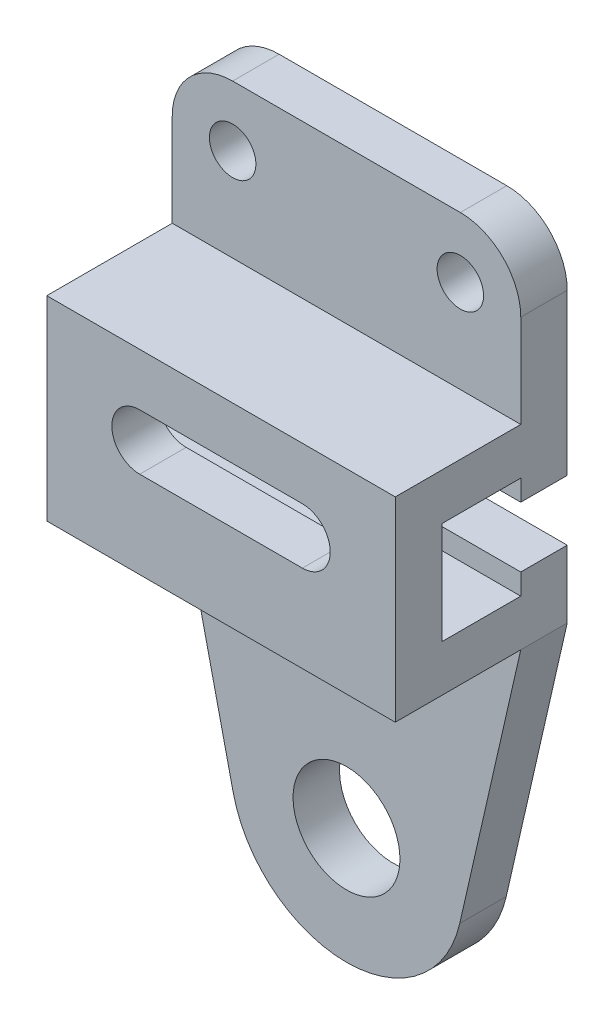
ISO-10303-21;
HEADER;
FILE_DESCRIPTION(('STEP AP214'),'2;1');
FILE_NAME('part.step','',(''),(''),'','','');
FILE_SCHEMA(('AUTOMOTIVE_DESIGN { 1 0 10303 214 1 1 1 1 }'));
ENDSEC;
DATA;
#1=APPLICATION_CONTEXT('core data for automotive mechanical design processes');
#2=APPLICATION_PROTOCOL_DEFINITION('international standard','automotive_design',2000,#1);
#3=PRODUCT_CONTEXT('',#1,'mechanical');
#4=PRODUCT('Part','Part','',(#3));
#5=PRODUCT_RELATED_PRODUCT_CATEGORY('part','',(#4));
#6=PRODUCT_DEFINITION_FORMATION('','',#4);
#7=PRODUCT_DEFINITION_CONTEXT('part definition',#1,'design');
#8=PRODUCT_DEFINITION('design','',#6,#7);
#9=PRODUCT_DEFINITION_SHAPE('','',#8);
#10=(LENGTH_UNIT() NAMED_UNIT(*) SI_UNIT(.MILLI.,.METRE.));
#11=(NAMED_UNIT(*) PLANE_ANGLE_UNIT() SI_UNIT($,.RADIAN.));
#12=(NAMED_UNIT(*) SI_UNIT($,.STERADIAN.) SOLID_ANGLE_UNIT());
#13=UNCERTAINTY_MEASURE_WITH_UNIT(LENGTH_MEASURE(1.E-05),#10,'distance_accuracy_value','');
#14=(GEOMETRIC_REPRESENTATION_CONTEXT(3) GLOBAL_UNCERTAINTY_ASSIGNED_CONTEXT((#13)) GLOBAL_UNIT_ASSIGNED_CONTEXT((#10,
#11,#12)) REPRESENTATION_CONTEXT('',''));
#15=CARTESIAN_POINT('',(0.,0.,0.));
#16=DIRECTION('',(0.,0.,1.));
#17=DIRECTION('',(1.,0.,0.));
#18=AXIS2_PLACEMENT_3D('',#15,#16,#17);
#19=CARTESIAN_POINT('',(0.,63.5,37.));
#20=DIRECTION('',(0.,1.,0.));
#21=DIRECTION('',(0.,0.,1.));
#22=AXIS2_PLACEMENT_3D('',#19,#20,#21);
#23=PLANE('',#22);
#24=DIRECTION('',(0.,0.,-1.));
#25=VECTOR('',#24,1.);
#26=CARTESIAN_POINT('',(-24.4999999999999,63.5,37.));
#27=LINE('',#26,#25);
#28=CARTESIAN_POINT('',(-24.5,63.5,10.));
#29=VERTEX_POINT('',#28);
#30=CARTESIAN_POINT('',(-24.4999999999999,63.5,0.));
#31=VERTEX_POINT('',#30);
#32=EDGE_CURVE('E319',#29,#31,#27,.T.);
#33=ORIENTED_EDGE('',*,*,#32,.F.);
#34=DIRECTION('',(1.,0.,0.));
#35=VECTOR('',#34,1.);
#36=CARTESIAN_POINT('',(-37.5,63.5,10.));
#37=LINE('',#36,#35);
#38=CARTESIAN_POINT('',(24.5,63.5,10.));
#39=VERTEX_POINT('',#38);
#40=EDGE_CURVE('E420',#29,#39,#37,.T.);
#41=ORIENTED_EDGE('',*,*,#40,.T.);
#42=DIRECTION('',(0.,0.,-1.));
#43=VECTOR('',#42,1.);
#44=CARTESIAN_POINT('',(24.4999999999999,63.5,37.));
#45=LINE('',#44,#43);
#46=CARTESIAN_POINT('',(24.4999999999999,63.5,0.));
#47=VERTEX_POINT('',#46);
#48=EDGE_CURVE('E301',#39,#47,#45,.T.);
#49=ORIENTED_EDGE('',*,*,#48,.T.);
#50=DIRECTION('',(1.,0.,0.));
#51=VECTOR('',#50,1.);
#52=CARTESIAN_POINT('',(0.,63.5,0.));
#53=LINE('',#52,#51);
#54=EDGE_CURVE('E277',#31,#47,#53,.T.);
#55=ORIENTED_EDGE('',*,*,#54,.F.);
#56=EDGE_LOOP('',(#33,#41,#49,#55));
#57=FACE_BOUND('',#56,.T.);
#58=ADVANCED_FACE('F41',(#57),#23,.T.);
#59=CARTESIAN_POINT('',(-37.5,0.,37.));
#60=DIRECTION('',(1.,0.,0.));
#61=DIRECTION('',(0.,1.,0.));
#62=AXIS2_PLACEMENT_3D('',#59,#60,#61);
#63=PLANE('',#62);
#64=DIRECTION('',(0.,0.,-1.));
#65=VECTOR('',#64,1.);
#66=CARTESIAN_POINT('',(-37.5,30.5,0.));
#67=LINE('',#66,#65);
#68=CARTESIAN_POINT('',(-37.5,30.5,37.));
#69=VERTEX_POINT('',#68);
#70=CARTESIAN_POINT('',(-37.5,30.5,10.));
#71=VERTEX_POINT('',#70);
#72=EDGE_CURVE('E226',#69,#71,#67,.T.);
#73=ORIENTED_EDGE('',*,*,#72,.T.);
#74=DIRECTION('',(0.,1.,0.));
#75=VECTOR('',#74,1.);
#76=CARTESIAN_POINT('',(-37.5,0.,10.));
#77=LINE('',#76,#75);
#78=CARTESIAN_POINT('',(-37.5,50.5,10.));
#79=VERTEX_POINT('',#78);
#80=EDGE_CURVE('E231',#71,#79,#77,.T.);
#81=ORIENTED_EDGE('',*,*,#80,.T.);
#82=DIRECTION('',(0.,0.,-1.));
#83=VECTOR('',#82,1.);
#84=CARTESIAN_POINT('',(-37.5,50.4999999999999,37.));
#85=LINE('',#84,#83);
#86=CARTESIAN_POINT('',(-37.5,50.4999999999999,0.));
#87=VERTEX_POINT('',#86);
#88=EDGE_CURVE('E318',#79,#87,#85,.T.);
#89=ORIENTED_EDGE('',*,*,#88,.T.);
#90=DIRECTION('',(0.,-1.,0.));
#91=VECTOR('',#90,1.);
#92=CARTESIAN_POINT('',(-37.5,0.,0.));
#93=LINE('',#92,#91);
#94=CARTESIAN_POINT('',(-37.5,16.,0.));
#95=VERTEX_POINT('',#94);
#96=EDGE_CURVE('E285',#87,#95,#93,.T.);
#97=ORIENTED_EDGE('',*,*,#96,.T.);
#98=DIRECTION('',(0.,0.,-1.));
#99=VECTOR('',#98,1.);
#100=CARTESIAN_POINT('',(-37.5,16.,0.));
#101=LINE('',#100,#99);
#102=CARTESIAN_POINT('',(-37.5,16.,10.));
#103=VERTEX_POINT('',#102);
#104=EDGE_CURVE('E457',#103,#95,#101,.T.);
#105=ORIENTED_EDGE('',*,*,#104,.F.);
#106=DIRECTION('',(0.,-1.,0.));
#107=VECTOR('',#106,1.);
#108=CARTESIAN_POINT('',(-37.5,0.,9.99999999999999));
#109=LINE('',#108,#107);
#110=CARTESIAN_POINT('',(-37.5,20.5,10.));
#111=VERTEX_POINT('',#110);
#112=EDGE_CURVE('E504',#111,#103,#109,.T.);
#113=ORIENTED_EDGE('',*,*,#112,.F.);
#114=DIRECTION('',(0.,0.,-1.));
#115=VECTOR('',#114,1.);
#116=CARTESIAN_POINT('',(-37.5,20.5,0.));
#117=LINE('',#116,#115);
#118=CARTESIAN_POINT('',(-37.5,20.5,27.));
#119=VERTEX_POINT('',#118);
#120=EDGE_CURVE('E482',#119,#111,#117,.T.);
#121=ORIENTED_EDGE('',*,*,#120,.F.);
#122=DIRECTION('',(0.,-1.,0.));
#123=VECTOR('',#122,1.);
#124=CARTESIAN_POINT('',(-37.5,0.,27.));
#125=LINE('',#124,#123);
#126=CARTESIAN_POINT('',(-37.5,-1.50000000000002,27.));
#127=VERTEX_POINT('',#126);
#128=EDGE_CURVE('E491',#119,#127,#125,.T.);
#129=ORIENTED_EDGE('',*,*,#128,.T.);
#130=DIRECTION('',(0.,0.,-1.));
#131=VECTOR('',#130,1.);
#132=CARTESIAN_POINT('',(-37.5,-1.50000000000002,0.));
#133=LINE('',#132,#131);
#134=CARTESIAN_POINT('',(-37.5,-1.50000000000002,10.));
#135=VERTEX_POINT('',#134);
#136=EDGE_CURVE('E493',#127,#135,#133,.T.);
#137=ORIENTED_EDGE('',*,*,#136,.T.);
#138=DIRECTION('',(0.,-1.,0.));
#139=VECTOR('',#138,1.);
#140=CARTESIAN_POINT('',(-37.5,0.,10.));
#141=LINE('',#140,#139);
#142=CARTESIAN_POINT('',(-37.5,2.99999999999998,10.));
#143=VERTEX_POINT('',#142);
#144=EDGE_CURVE('E500',#143,#135,#141,.T.);
#145=ORIENTED_EDGE('',*,*,#144,.F.);
#146=DIRECTION('',(0.,0.,-1.));
#147=VECTOR('',#146,1.);
#148=CARTESIAN_POINT('',(-37.5,2.99999999999998,0.));
#149=LINE('',#148,#147);
#150=CARTESIAN_POINT('',(-37.5,2.99999999999998,0.));
#151=VERTEX_POINT('',#150);
#152=EDGE_CURVE('E393',#143,#151,#149,.T.);
#153=ORIENTED_EDGE('',*,*,#152,.T.);
#154=CARTESIAN_POINT('',(-37.5,-11.5,0.));
#155=VERTEX_POINT('',#154);
#156=EDGE_CURVE('E281',#151,#155,#93,.T.);
#157=ORIENTED_EDGE('',*,*,#156,.T.);
#158=DIRECTION('',(0.,0.,-1.));
#159=VECTOR('',#158,1.);
#160=CARTESIAN_POINT('',(-37.5,-11.5,37.));
#161=LINE('',#160,#159);
#162=CARTESIAN_POINT('',(-37.5,-11.5,10.));
#163=VERTEX_POINT('',#162);
#164=EDGE_CURVE('E312',#163,#155,#161,.T.);
#165=ORIENTED_EDGE('',*,*,#164,.F.);
#166=CARTESIAN_POINT('',(-37.5,-11.5,37.));
#167=VERTEX_POINT('',#166);
#168=EDGE_CURVE('E316',#167,#163,#161,.T.);
#169=ORIENTED_EDGE('',*,*,#168,.F.);
#170=DIRECTION('',(0.,-1.,0.));
#171=VECTOR('',#170,1.);
#172=CARTESIAN_POINT('',(-37.5,0.,37.));
#173=LINE('',#172,#171);
#174=EDGE_CURVE('E249',#69,#167,#173,.T.);
#175=ORIENTED_EDGE('',*,*,#174,.F.);
#176=EDGE_LOOP('',(#73,#81,#89,#97,#105,#113,#121,#129,#137,#145,#153,#157,#165,#169,#175));
#177=FACE_BOUND('',#176,.T.);
#178=ADVANCED_FACE('F389',(#177),#63,.F.);
#179=CARTESIAN_POINT('',(17.5,13.2267970959292,37.));
#180=DIRECTION('',(0.,0.,-1.));
#181=DIRECTION('',(-1.,0.,0.));
#182=AXIS2_PLACEMENT_3D('',#179,#180,#181);
#183=CYLINDRICAL_SURFACE('',#182,6.00000000000001);
#184=DIRECTION('',(0.,0.,-1.));
#185=VECTOR('',#184,1.);
#186=CARTESIAN_POINT('',(22.8206527468774,16.,37.));
#187=LINE('',#186,#185);
#188=CARTESIAN_POINT('',(22.8206527468774,16.,0.));
#189=VERTEX_POINT('',#188);
#190=CARTESIAN_POINT('',(22.8206527468774,16.,10.));
#191=VERTEX_POINT('',#190);
#192=EDGE_CURVE('E416',#189,#191,#187,.F.);
#193=ORIENTED_EDGE('',*,*,#192,.T.);
#194=CARTESIAN_POINT('',(17.5,13.2267970959292,9.99999999999999));
#195=DIRECTION('',(0.,0.,1.));
#196=DIRECTION('',(0.,-1.,0.));
#197=AXIS2_PLACEMENT_3D('',#194,#195,#196);
#198=CIRCLE('',#197,6.00000000000001);
#199=CARTESIAN_POINT('',(17.5,19.2267970959292,10.));
#200=VERTEX_POINT('',#199);
#201=EDGE_CURVE('E373',#191,#200,#198,.T.);
#202=ORIENTED_EDGE('',*,*,#201,.T.);
#203=DIRECTION('',(0.,0.,-1.));
#204=VECTOR('',#203,1.);
#205=CARTESIAN_POINT('',(17.5,19.2267970959292,37.));
#206=LINE('',#205,#204);
#207=CARTESIAN_POINT('',(17.5,19.2267970959292,0.));
#208=VERTEX_POINT('',#207);
#209=EDGE_CURVE('E246',#200,#208,#206,.T.);
#210=ORIENTED_EDGE('',*,*,#209,.T.);
#211=CARTESIAN_POINT('',(17.5,13.2267970959292,0.));
#212=DIRECTION('',(0.,0.,1.));
#213=DIRECTION('',(1.,0.,0.));
#214=AXIS2_PLACEMENT_3D('',#211,#212,#213);
#215=CIRCLE('',#214,6.00000000000001);
#216=EDGE_CURVE('E260',#189,#208,#215,.T.);
#217=ORIENTED_EDGE('',*,*,#216,.F.);
#218=EDGE_LOOP('',(#193,#202,#210,#217));
#219=FACE_BOUND('',#218,.T.);
#220=ADVANCED_FACE('F542',(#219),#183,.F.);
#221=CARTESIAN_POINT('',(-17.5,13.2267970959292,37.));
#222=DIRECTION('',(0.,0.,-1.));
#223=DIRECTION('',(-1.,0.,0.));
#224=AXIS2_PLACEMENT_3D('',#221,#222,#223);
#225=CYLINDRICAL_SURFACE('',#224,6.00000000000001);
#226=DIRECTION('',(0.,0.,-1.));
#227=VECTOR('',#226,1.);
#228=CARTESIAN_POINT('',(-17.5,19.2267970959292,37.));
#229=LINE('',#228,#227);
#230=CARTESIAN_POINT('',(-17.5,19.2267970959292,10.));
#231=VERTEX_POINT('',#230);
#232=CARTESIAN_POINT('',(-17.5,19.2267970959292,0.));
#233=VERTEX_POINT('',#232);
#234=EDGE_CURVE('E322',#231,#233,#229,.T.);
#235=ORIENTED_EDGE('',*,*,#234,.F.);
#236=CARTESIAN_POINT('',(-17.5,13.2267970959292,9.99999999999999));
#237=DIRECTION('',(0.,0.,1.));
#238=DIRECTION('',(0.,-1.,0.));
#239=AXIS2_PLACEMENT_3D('',#236,#237,#238);
#240=CIRCLE('',#239,6.00000000000001);
#241=CARTESIAN_POINT('',(-22.8206527468774,16.,10.));
#242=VERTEX_POINT('',#241);
#243=EDGE_CURVE('E63',#231,#242,#240,.T.);
#244=ORIENTED_EDGE('',*,*,#243,.T.);
#245=DIRECTION('',(0.,0.,-1.));
#246=VECTOR('',#245,1.);
#247=CARTESIAN_POINT('',(-22.8206527468774,16.,37.));
#248=LINE('',#247,#246);
#249=CARTESIAN_POINT('',(-22.8206527468774,16.,0.));
#250=VERTEX_POINT('',#249);
#251=EDGE_CURVE('E412',#242,#250,#248,.T.);
#252=ORIENTED_EDGE('',*,*,#251,.T.);
#253=CARTESIAN_POINT('',(-17.5,13.2267970959292,0.));
#254=DIRECTION('',(0.,0.,1.));
#255=DIRECTION('',(1.,0.,0.));
#256=AXIS2_PLACEMENT_3D('',#253,#254,#255);
#257=CIRCLE('',#256,6.00000000000001);
#258=EDGE_CURVE('E257',#233,#250,#257,.T.);
#259=ORIENTED_EDGE('',*,*,#258,.F.);
#260=EDGE_LOOP('',(#235,#244,#252,#259));
#261=FACE_BOUND('',#260,.T.);
#262=ADVANCED_FACE('F549',(#261),#225,.F.);
#263=CARTESIAN_POINT('',(0.,19.2267970959292,37.));
#264=DIRECTION('',(0.,1.,0.));
#265=DIRECTION('',(-1.,0.,0.));
#266=AXIS2_PLACEMENT_3D('',#263,#264,#265);
#267=PLANE('',#266);
#268=DIRECTION('',(1.,0.,0.));
#269=VECTOR('',#268,1.);
#270=CARTESIAN_POINT('',(0.,19.2267970959292,10.));
#271=LINE('',#270,#269);
#272=EDGE_CURVE('E11',#231,#200,#271,.T.);
#273=ORIENTED_EDGE('',*,*,#272,.F.);
#274=ORIENTED_EDGE('',*,*,#234,.T.);
#275=DIRECTION('',(1.,0.,0.));
#276=VECTOR('',#275,1.);
#277=CARTESIAN_POINT('',(0.,19.2267970959292,0.));
#278=LINE('',#277,#276);
#279=EDGE_CURVE('E262',#233,#208,#278,.T.);
#280=ORIENTED_EDGE('',*,*,#279,.T.);
#281=ORIENTED_EDGE('',*,*,#209,.F.);
#282=EDGE_LOOP('',(#273,#274,#280,#281));
#283=FACE_BOUND('',#282,.T.);
#284=ADVANCED_FACE('F550',(#283),#267,.F.);
#285=CARTESIAN_POINT('',(0.,0.,37.));
#286=DIRECTION('',(0.,0.,1.));
#287=DIRECTION('',(1.,0.,0.));
#288=AXIS2_PLACEMENT_3D('',#285,#286,#287);
#289=PLANE('',#288);
#290=DIRECTION('',(1.,0.,0.));
#291=VECTOR('',#290,1.);
#292=CARTESIAN_POINT('',(-37.5,30.5,37.));
#293=LINE('',#292,#291);
#294=CARTESIAN_POINT('',(37.5,30.5,37.));
#295=VERTEX_POINT('',#294);
#296=EDGE_CURVE('E222',#69,#295,#293,.T.);
#297=ORIENTED_EDGE('',*,*,#296,.F.);
#298=ORIENTED_EDGE('',*,*,#174,.T.);
#299=DIRECTION('',(1.,0.,0.));
#300=VECTOR('',#299,1.);
#301=CARTESIAN_POINT('',(-37.5,-11.5,37.));
#302=LINE('',#301,#300);
#303=CARTESIAN_POINT('',(37.5,-11.5,37.));
#304=VERTEX_POINT('',#303);
#305=EDGE_CURVE('E250',#167,#304,#302,.T.);
#306=ORIENTED_EDGE('',*,*,#305,.T.);
#307=DIRECTION('',(0.,-1.,0.));
#308=VECTOR('',#307,1.);
#309=CARTESIAN_POINT('',(37.5,0.,37.));
#310=LINE('',#309,#308);
#311=EDGE_CURVE('E239',#295,#304,#310,.T.);
#312=ORIENTED_EDGE('',*,*,#311,.F.);
#313=EDGE_LOOP('',(#297,#298,#306,#312));
#314=FACE_BOUND('',#313,.T.);
#315=CARTESIAN_POINT('',(17.5,13.2267970959292,37.));
#316=DIRECTION('',(0.,0.,1.));
#317=DIRECTION('',(1.,0.,0.));
#318=AXIS2_PLACEMENT_3D('',#315,#316,#317);
#319=CIRCLE('',#318,6.00000000000001);
#320=CARTESIAN_POINT('',(17.5,7.22679709592923,37.));
#321=VERTEX_POINT('',#320);
#322=CARTESIAN_POINT('',(17.5,19.2267970959292,37.));
#323=VERTEX_POINT('',#322);
#324=EDGE_CURVE('E305',#321,#323,#319,.T.);
#325=ORIENTED_EDGE('',*,*,#324,.F.);
#326=DIRECTION('',(1.,0.,0.));
#327=VECTOR('',#326,1.);
#328=CARTESIAN_POINT('',(0.,7.22679709592923,37.));
#329=LINE('',#328,#327);
#330=CARTESIAN_POINT('',(-17.5,7.22679709592923,37.));
#331=VERTEX_POINT('',#330);
#332=EDGE_CURVE('E349',#331,#321,#329,.T.);
#333=ORIENTED_EDGE('',*,*,#332,.F.);
#334=CARTESIAN_POINT('',(-17.5,13.2267970959292,37.));
#335=DIRECTION('',(0.,0.,1.));
#336=DIRECTION('',(1.,0.,0.));
#337=AXIS2_PLACEMENT_3D('',#334,#335,#336);
#338=CIRCLE('',#337,6.00000000000001);
#339=CARTESIAN_POINT('',(-17.5,19.2267970959292,37.));
#340=VERTEX_POINT('',#339);
#341=EDGE_CURVE('E354',#340,#331,#338,.T.);
#342=ORIENTED_EDGE('',*,*,#341,.F.);
#343=DIRECTION('',(1.,0.,0.));
#344=VECTOR('',#343,1.);
#345=CARTESIAN_POINT('',(0.,19.2267970959292,37.));
#346=LINE('',#345,#344);
#347=EDGE_CURVE('E251',#340,#323,#346,.T.);
#348=ORIENTED_EDGE('',*,*,#347,.T.);
#349=EDGE_LOOP('',(#325,#333,#342,#348));
#350=FACE_BOUND('',#349,.T.);
#351=ADVANCED_FACE('F242',(#314,#350),#289,.T.);
#352=CARTESIAN_POINT('',(0.,0.,0.));
#353=DIRECTION('',(0.,0.,1.));
#354=DIRECTION('',(1.,0.,0.));
#355=AXIS2_PLACEMENT_3D('',#352,#353,#354);
#356=PLANE('',#355);
#357=CARTESIAN_POINT('',(24.5,50.5,0.));
#358=DIRECTION('',(0.,0.,1.));
#359=DIRECTION('',(1.,0.,0.));
#360=AXIS2_PLACEMENT_3D('',#357,#358,#359);
#361=CIRCLE('',#360,5.);
#362=CARTESIAN_POINT('',(29.5,50.5,0.));
#363=VERTEX_POINT('',#362);
#364=EDGE_CURVE('E270',#363,#363,#361,.T.);
#365=ORIENTED_EDGE('',*,*,#364,.T.);
#366=EDGE_LOOP('',(#365));
#367=FACE_BOUND('',#366,.T.);
#368=CARTESIAN_POINT('',(-24.5,50.5,0.));
#369=DIRECTION('',(0.,0.,1.));
#370=DIRECTION('',(1.,0.,0.));
#371=AXIS2_PLACEMENT_3D('',#368,#369,#370);
#372=CIRCLE('',#371,5.);
#373=CARTESIAN_POINT('',(-19.5,50.5,0.));
#374=VERTEX_POINT('',#373);
#375=EDGE_CURVE('E269',#374,#374,#372,.T.);
#376=ORIENTED_EDGE('',*,*,#375,.T.);
#377=EDGE_LOOP('',(#376));
#378=FACE_BOUND('',#377,.T.);
#379=DIRECTION('',(1.,0.,0.));
#380=VECTOR('',#379,1.);
#381=CARTESIAN_POINT('',(-37.5,16.,0.));
#382=LINE('',#381,#380);
#383=EDGE_CURVE('E449',#95,#250,#382,.T.);
#384=ORIENTED_EDGE('',*,*,#383,.F.);
#385=ORIENTED_EDGE('',*,*,#96,.F.);
#386=CARTESIAN_POINT('',(-24.5,50.5,0.));
#387=DIRECTION('',(0.,0.,1.));
#388=DIRECTION('',(1.,0.,0.));
#389=AXIS2_PLACEMENT_3D('',#386,#387,#388);
#390=CIRCLE('',#389,13.);
#391=EDGE_CURVE('E276',#31,#87,#390,.T.);
#392=ORIENTED_EDGE('',*,*,#391,.F.);
#393=ORIENTED_EDGE('',*,*,#54,.T.);
#394=CARTESIAN_POINT('',(24.5,50.5,0.));
#395=DIRECTION('',(0.,0.,1.));
#396=DIRECTION('',(1.,0.,0.));
#397=AXIS2_PLACEMENT_3D('',#394,#395,#396);
#398=CIRCLE('',#397,13.);
#399=CARTESIAN_POINT('',(37.5,50.4999999999999,0.));
#400=VERTEX_POINT('',#399);
#401=EDGE_CURVE('E298',#47,#400,#398,.F.);
#402=ORIENTED_EDGE('',*,*,#401,.T.);
#403=DIRECTION('',(0.,-1.,0.));
#404=VECTOR('',#403,1.);
#405=CARTESIAN_POINT('',(37.5,0.,0.));
#406=LINE('',#405,#404);
#407=CARTESIAN_POINT('',(37.5,16.,0.));
#408=VERTEX_POINT('',#407);
#409=EDGE_CURVE('E299',#400,#408,#406,.T.);
#410=ORIENTED_EDGE('',*,*,#409,.T.);
#411=EDGE_CURVE('E321',#189,#408,#382,.T.);
#412=ORIENTED_EDGE('',*,*,#411,.F.);
#413=ORIENTED_EDGE('',*,*,#216,.T.);
#414=ORIENTED_EDGE('',*,*,#279,.F.);
#415=ORIENTED_EDGE('',*,*,#258,.T.);
#416=EDGE_LOOP('',(#384,#385,#392,#393,#402,#410,#412,#413,#414,#415));
#417=FACE_BOUND('',#416,.T.);
#418=ADVANCED_FACE('F437',(#367,#378,#417),#356,.F.);
#419=CARTESIAN_POINT('',(-24.5,50.5,37.));
#420=DIRECTION('',(0.,0.,-1.));
#421=DIRECTION('',(-1.,0.,0.));
#422=AXIS2_PLACEMENT_3D('',#419,#420,#421);
#423=CYLINDRICAL_SURFACE('',#422,13.);
#424=ORIENTED_EDGE('',*,*,#88,.F.);
#425=CARTESIAN_POINT('',(-24.5,50.5,10.));
#426=DIRECTION('',(0.,0.,-1.));
#427=DIRECTION('',(0.,1.,0.));
#428=AXIS2_PLACEMENT_3D('',#425,#426,#427);
#429=CIRCLE('',#428,13.);
#430=EDGE_CURVE('E361',#79,#29,#429,.T.);
#431=ORIENTED_EDGE('',*,*,#430,.T.);
#432=ORIENTED_EDGE('',*,*,#32,.T.);
#433=ORIENTED_EDGE('',*,*,#391,.T.);
#434=EDGE_LOOP('',(#424,#431,#432,#433));
#435=FACE_BOUND('',#434,.T.);
#436=ADVANCED_FACE('F442',(#435),#423,.T.);
#437=CARTESIAN_POINT('',(-38.1391266227549,-8.69733249002864,37.));
#438=DIRECTION('',(0.974970454363625,0.222334462281461,0.));
#439=DIRECTION('',(-0.222334462281461,0.974970454363625,0.));
#440=AXIS2_PLACEMENT_3D('',#437,#438,#439);
#441=PLANE('',#440);
#442=DIRECTION('',(0.,0.,-1.));
#443=VECTOR('',#442,1.);
#444=CARTESIAN_POINT('',(-24.3742613590906,-69.0583615570365,37.));
#445=LINE('',#444,#443);
#446=CARTESIAN_POINT('',(-24.3742613590906,-69.0583615570365,10.));
#447=VERTEX_POINT('',#446);
#448=CARTESIAN_POINT('',(-24.3742613590906,-69.0583615570365,0.));
#449=VERTEX_POINT('',#448);
#450=EDGE_CURVE('E311',#447,#449,#445,.T.);
#451=ORIENTED_EDGE('',*,*,#450,.F.);
#452=DIRECTION('',(-0.222334462281461,0.974970454363625,0.));
#453=VECTOR('',#452,1.);
#454=CARTESIAN_POINT('',(-38.1391266227549,-8.69733249002864,10.));
#455=LINE('',#454,#453);
#456=EDGE_CURVE('E261',#447,#163,#455,.T.);
#457=ORIENTED_EDGE('',*,*,#456,.T.);
#458=ORIENTED_EDGE('',*,*,#164,.T.);
#459=DIRECTION('',(0.222334462281461,-0.974970454363625,0.));
#460=VECTOR('',#459,1.);
#461=CARTESIAN_POINT('',(-38.1391266227549,-8.69733249002864,0.));
#462=LINE('',#461,#460);
#463=EDGE_CURVE('E288',#155,#449,#462,.T.);
#464=ORIENTED_EDGE('',*,*,#463,.T.);
#465=EDGE_LOOP('',(#451,#457,#458,#464));
#466=FACE_BOUND('',#465,.T.);
#467=ADVANCED_FACE('F382',(#466),#441,.F.);
#468=CARTESIAN_POINT('',(0.,-63.5,37.));
#469=DIRECTION('',(0.,0.,-1.));
#470=DIRECTION('',(-1.,0.,0.));
#471=AXIS2_PLACEMENT_3D('',#468,#469,#470);
#472=CYLINDRICAL_SURFACE('',#471,25.);
#473=DIRECTION('',(0.,0.,-1.));
#474=VECTOR('',#473,1.);
#475=CARTESIAN_POINT('',(24.3742613590907,-69.0583615570365,37.));
#476=LINE('',#475,#474);
#477=CARTESIAN_POINT('',(24.3742613590907,-69.0583615570365,10.));
#478=VERTEX_POINT('',#477);
#479=CARTESIAN_POINT('',(24.3742613590907,-69.0583615570365,0.));
#480=VERTEX_POINT('',#479);
#481=EDGE_CURVE('E313',#478,#480,#476,.T.);
#482=ORIENTED_EDGE('',*,*,#481,.F.);
#483=CARTESIAN_POINT('',(0.,-63.5,10.));
#484=DIRECTION('',(0.,0.,-1.));
#485=DIRECTION('',(0.,1.,0.));
#486=AXIS2_PLACEMENT_3D('',#483,#484,#485);
#487=CIRCLE('',#486,25.);
#488=EDGE_CURVE('E60',#478,#447,#487,.T.);
#489=ORIENTED_EDGE('',*,*,#488,.T.);
#490=ORIENTED_EDGE('',*,*,#450,.T.);
#491=CARTESIAN_POINT('',(0.,-63.5,0.));
#492=DIRECTION('',(0.,0.,1.));
#493=DIRECTION('',(1.,0.,0.));
#494=AXIS2_PLACEMENT_3D('',#491,#492,#493);
#495=CIRCLE('',#494,25.);
#496=EDGE_CURVE('E289',#449,#480,#495,.T.);
#497=ORIENTED_EDGE('',*,*,#496,.T.);
#498=EDGE_LOOP('',(#482,#489,#490,#497));
#499=FACE_BOUND('',#498,.T.);
#500=ADVANCED_FACE('F402',(#499),#472,.T.);
#501=CARTESIAN_POINT('',(38.1391266227549,-8.6973324900286,37.));
#502=DIRECTION('',(-0.974970454363625,0.22233446228146,0.));
#503=DIRECTION('',(-0.22233446228146,-0.974970454363625,0.));
#504=AXIS2_PLACEMENT_3D('',#501,#502,#503);
#505=PLANE('',#504);
#506=DIRECTION('',(0.,0.,-1.));
#507=VECTOR('',#506,1.);
#508=CARTESIAN_POINT('',(37.5,-11.5,37.));
#509=LINE('',#508,#507);
#510=CARTESIAN_POINT('',(37.5,-11.5,10.));
#511=VERTEX_POINT('',#510);
#512=CARTESIAN_POINT('',(37.5,-11.5,0.));
#513=VERTEX_POINT('',#512);
#514=EDGE_CURVE('E306',#511,#513,#509,.T.);
#515=ORIENTED_EDGE('',*,*,#514,.F.);
#516=DIRECTION('',(-0.22233446228146,-0.974970454363625,0.));
#517=VECTOR('',#516,1.);
#518=CARTESIAN_POINT('',(38.1391266227549,-8.6973324900286,10.));
#519=LINE('',#518,#517);
#520=EDGE_CURVE('E376',#511,#478,#519,.T.);
#521=ORIENTED_EDGE('',*,*,#520,.T.);
#522=ORIENTED_EDGE('',*,*,#481,.T.);
#523=DIRECTION('',(0.22233446228146,0.974970454363626,0.));
#524=VECTOR('',#523,1.);
#525=CARTESIAN_POINT('',(38.1391266227549,-8.6973324900286,0.));
#526=LINE('',#525,#524);
#527=EDGE_CURVE('E295',#480,#513,#526,.T.);
#528=ORIENTED_EDGE('',*,*,#527,.T.);
#529=EDGE_LOOP('',(#515,#521,#522,#528));
#530=FACE_BOUND('',#529,.T.);
#531=ADVANCED_FACE('F404',(#530),#505,.F.);
#532=CARTESIAN_POINT('',(37.5,0.,37.));
#533=DIRECTION('',(1.,0.,0.));
#534=DIRECTION('',(0.,1.,0.));
#535=AXIS2_PLACEMENT_3D('',#532,#533,#534);
#536=PLANE('',#535);
#537=DIRECTION('',(0.,0.,-1.));
#538=VECTOR('',#537,1.);
#539=CARTESIAN_POINT('',(37.5,30.5,0.));
#540=LINE('',#539,#538);
#541=CARTESIAN_POINT('',(37.5,30.5,10.));
#542=VERTEX_POINT('',#541);
#543=EDGE_CURVE('E221',#295,#542,#540,.T.);
#544=ORIENTED_EDGE('',*,*,#543,.F.);
#545=ORIENTED_EDGE('',*,*,#311,.T.);
#546=EDGE_CURVE('E310',#304,#511,#509,.T.);
#547=ORIENTED_EDGE('',*,*,#546,.T.);
#548=ORIENTED_EDGE('',*,*,#514,.T.);
#549=CARTESIAN_POINT('',(37.5,2.99999999999998,0.));
#550=VERTEX_POINT('',#549);
#551=EDGE_CURVE('E293',#550,#513,#406,.T.);
#552=ORIENTED_EDGE('',*,*,#551,.F.);
#553=DIRECTION('',(0.,0.,-1.));
#554=VECTOR('',#553,1.);
#555=CARTESIAN_POINT('',(37.5,2.99999999999998,0.));
#556=LINE('',#555,#554);
#557=CARTESIAN_POINT('',(37.5,2.99999999999998,10.));
#558=VERTEX_POINT('',#557);
#559=EDGE_CURVE('E485',#558,#550,#556,.T.);
#560=ORIENTED_EDGE('',*,*,#559,.F.);
#561=DIRECTION('',(0.,-1.,0.));
#562=VECTOR('',#561,1.);
#563=CARTESIAN_POINT('',(37.5,0.,10.));
#564=LINE('',#563,#562);
#565=CARTESIAN_POINT('',(37.5,-1.50000000000002,10.));
#566=VERTEX_POINT('',#565);
#567=EDGE_CURVE('E486',#558,#566,#564,.T.);
#568=ORIENTED_EDGE('',*,*,#567,.T.);
#569=DIRECTION('',(0.,0.,-1.));
#570=VECTOR('',#569,1.);
#571=CARTESIAN_POINT('',(37.5,-1.50000000000002,0.));
#572=LINE('',#571,#570);
#573=CARTESIAN_POINT('',(37.5,-1.50000000000002,27.));
#574=VERTEX_POINT('',#573);
#575=EDGE_CURVE('E526',#574,#566,#572,.T.);
#576=ORIENTED_EDGE('',*,*,#575,.F.);
#577=DIRECTION('',(0.,-1.,0.));
#578=VECTOR('',#577,1.);
#579=CARTESIAN_POINT('',(37.5,0.,27.));
#580=LINE('',#579,#578);
#581=CARTESIAN_POINT('',(37.5,20.5,27.));
#582=VERTEX_POINT('',#581);
#583=EDGE_CURVE('E518',#582,#574,#580,.T.);
#584=ORIENTED_EDGE('',*,*,#583,.F.);
#585=DIRECTION('',(0.,0.,-1.));
#586=VECTOR('',#585,1.);
#587=CARTESIAN_POINT('',(37.5,20.5,0.));
#588=LINE('',#587,#586);
#589=CARTESIAN_POINT('',(37.5,20.5,10.));
#590=VERTEX_POINT('',#589);
#591=EDGE_CURVE('E413',#582,#590,#588,.T.);
#592=ORIENTED_EDGE('',*,*,#591,.T.);
#593=DIRECTION('',(0.,-1.,0.));
#594=VECTOR('',#593,1.);
#595=CARTESIAN_POINT('',(37.5,0.,9.99999999999999));
#596=LINE('',#595,#594);
#597=CARTESIAN_POINT('',(37.5,16.,10.));
#598=VERTEX_POINT('',#597);
#599=EDGE_CURVE('E479',#590,#598,#596,.T.);
#600=ORIENTED_EDGE('',*,*,#599,.T.);
#601=DIRECTION('',(0.,0.,-1.));
#602=VECTOR('',#601,1.);
#603=CARTESIAN_POINT('',(37.5,16.,0.));
#604=LINE('',#603,#602);
#605=EDGE_CURVE('E478',#598,#408,#604,.T.);
#606=ORIENTED_EDGE('',*,*,#605,.T.);
#607=ORIENTED_EDGE('',*,*,#409,.F.);
#608=DIRECTION('',(0.,0.,-1.));
#609=VECTOR('',#608,1.);
#610=CARTESIAN_POINT('',(37.5,50.4999999999999,37.));
#611=LINE('',#610,#609);
#612=CARTESIAN_POINT('',(37.5,50.4999999999999,10.));
#613=VERTEX_POINT('',#612);
#614=EDGE_CURVE('E302',#613,#400,#611,.T.);
#615=ORIENTED_EDGE('',*,*,#614,.F.);
#616=DIRECTION('',(0.,1.,0.));
#617=VECTOR('',#616,1.);
#618=CARTESIAN_POINT('',(37.5,0.,10.));
#619=LINE('',#618,#617);
#620=EDGE_CURVE('E244',#542,#613,#619,.T.);
#621=ORIENTED_EDGE('',*,*,#620,.F.);
#622=EDGE_LOOP('',(#544,#545,#547,#548,#552,#560,#568,#576,#584,#592,#600,#606,#607,#615,#621));
#623=FACE_BOUND('',#622,.T.);
#624=ADVANCED_FACE('F240',(#623),#536,.T.);
#625=CARTESIAN_POINT('',(17.5,13.2267970959292,27.));
#626=DIRECTION('',(0.,0.,1.));
#627=DIRECTION('',(1.,0.,0.));
#628=AXIS2_PLACEMENT_3D('',#625,#626,#627);
#629=CIRCLE('',#628,6.00000000000001);
#630=CARTESIAN_POINT('',(17.5,7.22679709592923,27.));
#631=VERTEX_POINT('',#630);
#632=CARTESIAN_POINT('',(17.5,19.2267970959292,27.));
#633=VERTEX_POINT('',#632);
#634=EDGE_CURVE('E342',#631,#633,#629,.T.);
#635=ORIENTED_EDGE('',*,*,#634,.F.);
#636=DIRECTION('',(0.,0.,-1.));
#637=VECTOR('',#636,1.);
#638=CARTESIAN_POINT('',(17.5,7.22679709592923,37.));
#639=LINE('',#638,#637);
#640=EDGE_CURVE('E308',#321,#631,#639,.T.);
#641=ORIENTED_EDGE('',*,*,#640,.F.);
#642=ORIENTED_EDGE('',*,*,#324,.T.);
#643=EDGE_CURVE('E253',#323,#633,#206,.T.);
#644=ORIENTED_EDGE('',*,*,#643,.T.);
#645=EDGE_LOOP('',(#635,#641,#642,#644));
#646=FACE_BOUND('',#645,.T.);
#647=ADVANCED_FACE('F43',(#646),#183,.F.);
#648=CARTESIAN_POINT('',(0.,7.22679709592923,37.));
#649=DIRECTION('',(0.,1.,0.));
#650=DIRECTION('',(-1.,0.,0.));
#651=AXIS2_PLACEMENT_3D('',#648,#649,#650);
#652=PLANE('',#651);
#653=DIRECTION('',(1.,0.,0.));
#654=VECTOR('',#653,1.);
#655=CARTESIAN_POINT('',(0.,7.22679709592923,27.));
#656=LINE('',#655,#654);
#657=CARTESIAN_POINT('',(-17.5,7.22679709592923,27.));
#658=VERTEX_POINT('',#657);
#659=EDGE_CURVE('E362',#658,#631,#656,.T.);
#660=ORIENTED_EDGE('',*,*,#659,.F.);
#661=DIRECTION('',(0.,0.,-1.));
#662=VECTOR('',#661,1.);
#663=CARTESIAN_POINT('',(-17.5,7.22679709592923,37.));
#664=LINE('',#663,#662);
#665=EDGE_CURVE('E327',#331,#658,#664,.T.);
#666=ORIENTED_EDGE('',*,*,#665,.F.);
#667=ORIENTED_EDGE('',*,*,#332,.T.);
#668=ORIENTED_EDGE('',*,*,#640,.T.);
#669=EDGE_LOOP('',(#660,#666,#667,#668));
#670=FACE_BOUND('',#669,.T.);
#671=ADVANCED_FACE('F577',(#670),#652,.T.);
#672=CARTESIAN_POINT('',(-17.5,13.2267970959292,27.));
#673=DIRECTION('',(0.,0.,1.));
#674=DIRECTION('',(1.,0.,0.));
#675=AXIS2_PLACEMENT_3D('',#672,#673,#674);
#676=CIRCLE('',#675,6.00000000000001);
#677=CARTESIAN_POINT('',(-17.5,19.2267970959292,27.));
#678=VERTEX_POINT('',#677);
#679=EDGE_CURVE('E357',#678,#658,#676,.T.);
#680=ORIENTED_EDGE('',*,*,#679,.F.);
#681=EDGE_CURVE('E324',#340,#678,#229,.T.);
#682=ORIENTED_EDGE('',*,*,#681,.F.);
#683=ORIENTED_EDGE('',*,*,#341,.T.);
#684=ORIENTED_EDGE('',*,*,#665,.T.);
#685=EDGE_LOOP('',(#680,#682,#683,#684));
#686=FACE_BOUND('',#685,.T.);
#687=ADVANCED_FACE('F359',(#686),#225,.F.);
#688=CARTESIAN_POINT('',(0.,-63.5,37.));
#689=DIRECTION('',(0.,0.,-1.));
#690=DIRECTION('',(-1.,0.,0.));
#691=AXIS2_PLACEMENT_3D('',#688,#689,#690);
#692=CYLINDRICAL_SURFACE('',#691,11.5);
#693=CARTESIAN_POINT('',(0.,-63.5,10.));
#694=DIRECTION('',(0.,0.,-1.));
#695=DIRECTION('',(0.,1.,0.));
#696=AXIS2_PLACEMENT_3D('',#693,#694,#695);
#697=CIRCLE('',#696,11.5);
#698=CARTESIAN_POINT('',(0.,-52.,10.));
#699=VERTEX_POINT('',#698);
#700=EDGE_CURVE('E44',#699,#699,#697,.T.);
#701=ORIENTED_EDGE('',*,*,#700,.F.);
#702=EDGE_LOOP('',(#701));
#703=FACE_BOUND('',#702,.T.);
#704=CARTESIAN_POINT('',(0.,-63.5,0.));
#705=DIRECTION('',(0.,0.,1.));
#706=DIRECTION('',(1.,0.,0.));
#707=AXIS2_PLACEMENT_3D('',#704,#705,#706);
#708=CIRCLE('',#707,11.5);
#709=CARTESIAN_POINT('',(11.5,-63.5,0.));
#710=VERTEX_POINT('',#709);
#711=EDGE_CURVE('E272',#710,#710,#708,.T.);
#712=ORIENTED_EDGE('',*,*,#711,.F.);
#713=EDGE_LOOP('',(#712));
#714=FACE_BOUND('',#713,.T.);
#715=ADVANCED_FACE('F432',(#703,#714),#692,.F.);
#716=CARTESIAN_POINT('',(-24.5,50.5,37.));
#717=DIRECTION('',(0.,0.,-1.));
#718=DIRECTION('',(-1.,0.,0.));
#719=AXIS2_PLACEMENT_3D('',#716,#717,#718);
#720=CYLINDRICAL_SURFACE('',#719,5.);
#721=CARTESIAN_POINT('',(-24.5,50.5,10.));
#722=DIRECTION('',(0.,0.,-1.));
#723=DIRECTION('',(0.,1.,0.));
#724=AXIS2_PLACEMENT_3D('',#721,#722,#723);
#725=CIRCLE('',#724,5.);
#726=CARTESIAN_POINT('',(-24.5,55.5,10.));
#727=VERTEX_POINT('',#726);
#728=EDGE_CURVE('E370',#727,#727,#725,.T.);
#729=ORIENTED_EDGE('',*,*,#728,.F.);
#730=EDGE_LOOP('',(#729));
#731=FACE_BOUND('',#730,.T.);
#732=ORIENTED_EDGE('',*,*,#375,.F.);
#733=EDGE_LOOP('',(#732));
#734=FACE_BOUND('',#733,.T.);
#735=ADVANCED_FACE('F429',(#731,#734),#720,.F.);
#736=CARTESIAN_POINT('',(24.5,50.5,37.));
#737=DIRECTION('',(0.,0.,-1.));
#738=DIRECTION('',(-1.,0.,0.));
#739=AXIS2_PLACEMENT_3D('',#736,#737,#738);
#740=CYLINDRICAL_SURFACE('',#739,5.);
#741=CARTESIAN_POINT('',(24.5,50.5,10.));
#742=DIRECTION('',(0.,0.,-1.));
#743=DIRECTION('',(0.,1.,0.));
#744=AXIS2_PLACEMENT_3D('',#741,#742,#743);
#745=CIRCLE('',#744,5.);
#746=CARTESIAN_POINT('',(24.5,55.5,10.));
#747=VERTEX_POINT('',#746);
#748=EDGE_CURVE('E425',#747,#747,#745,.T.);
#749=ORIENTED_EDGE('',*,*,#748,.F.);
#750=EDGE_LOOP('',(#749));
#751=FACE_BOUND('',#750,.T.);
#752=ORIENTED_EDGE('',*,*,#364,.F.);
#753=EDGE_LOOP('',(#752));
#754=FACE_BOUND('',#753,.T.);
#755=ADVANCED_FACE('F433',(#751,#754),#740,.F.);
#756=ORIENTED_EDGE('',*,*,#681,.T.);
#757=DIRECTION('',(1.,0.,0.));
#758=VECTOR('',#757,1.);
#759=CARTESIAN_POINT('',(0.,19.2267970959292,27.));
#760=LINE('',#759,#758);
#761=EDGE_CURVE('E49',#678,#633,#760,.T.);
#762=ORIENTED_EDGE('',*,*,#761,.T.);
#763=ORIENTED_EDGE('',*,*,#643,.F.);
#764=ORIENTED_EDGE('',*,*,#347,.F.);
#765=EDGE_LOOP('',(#756,#762,#763,#764));
#766=FACE_BOUND('',#765,.T.);
#767=ADVANCED_FACE('F340',(#766),#267,.F.);
#768=CARTESIAN_POINT('',(24.5,50.5,37.));
#769=DIRECTION('',(0.,0.,-1.));
#770=DIRECTION('',(-1.,0.,0.));
#771=AXIS2_PLACEMENT_3D('',#768,#769,#770);
#772=CYLINDRICAL_SURFACE('',#771,13.);
#773=CARTESIAN_POINT('',(24.5,50.5,10.));
#774=DIRECTION('',(0.,0.,-1.));
#775=DIRECTION('',(0.,1.,0.));
#776=AXIS2_PLACEMENT_3D('',#773,#774,#775);
#777=CIRCLE('',#776,13.);
#778=EDGE_CURVE('E334',#613,#39,#777,.F.);
#779=ORIENTED_EDGE('',*,*,#778,.F.);
#780=ORIENTED_EDGE('',*,*,#614,.T.);
#781=ORIENTED_EDGE('',*,*,#401,.F.);
#782=ORIENTED_EDGE('',*,*,#48,.F.);
#783=EDGE_LOOP('',(#779,#780,#781,#782));
#784=FACE_BOUND('',#783,.T.);
#785=ADVANCED_FACE('F469',(#784),#772,.T.);
#786=ORIENTED_EDGE('',*,*,#711,.T.);
#787=EDGE_LOOP('',(#786));
#788=FACE_BOUND('',#787,.T.);
#789=ORIENTED_EDGE('',*,*,#156,.F.);
#790=DIRECTION('',(1.,0.,0.));
#791=VECTOR('',#790,1.);
#792=CARTESIAN_POINT('',(-37.5,2.99999999999998,0.));
#793=LINE('',#792,#791);
#794=EDGE_CURVE('E455',#151,#550,#793,.T.);
#795=ORIENTED_EDGE('',*,*,#794,.T.);
#796=ORIENTED_EDGE('',*,*,#551,.T.);
#797=ORIENTED_EDGE('',*,*,#527,.F.);
#798=ORIENTED_EDGE('',*,*,#496,.F.);
#799=ORIENTED_EDGE('',*,*,#463,.F.);
#800=EDGE_LOOP('',(#789,#795,#796,#797,#798,#799));
#801=FACE_BOUND('',#800,.T.);
#802=ADVANCED_FACE('F396',(#788,#801),#356,.F.);
#803=CARTESIAN_POINT('',(-37.5,0.,10.));
#804=DIRECTION('',(0.,0.,-1.));
#805=DIRECTION('',(0.,1.,0.));
#806=AXIS2_PLACEMENT_3D('',#803,#804,#805);
#807=PLANE('',#806);
#808=ORIENTED_EDGE('',*,*,#728,.T.);
#809=EDGE_LOOP('',(#808));
#810=FACE_BOUND('',#809,.T.);
#811=ORIENTED_EDGE('',*,*,#748,.T.);
#812=EDGE_LOOP('',(#811));
#813=FACE_BOUND('',#812,.T.);
#814=ORIENTED_EDGE('',*,*,#80,.F.);
#815=DIRECTION('',(1.,0.,0.));
#816=VECTOR('',#815,1.);
#817=CARTESIAN_POINT('',(-37.5,30.5,10.));
#818=LINE('',#817,#816);
#819=EDGE_CURVE('E235',#71,#542,#818,.T.);
#820=ORIENTED_EDGE('',*,*,#819,.T.);
#821=ORIENTED_EDGE('',*,*,#620,.T.);
#822=ORIENTED_EDGE('',*,*,#778,.T.);
#823=ORIENTED_EDGE('',*,*,#40,.F.);
#824=ORIENTED_EDGE('',*,*,#430,.F.);
#825=EDGE_LOOP('',(#814,#820,#821,#822,#823,#824));
#826=FACE_BOUND('',#825,.T.);
#827=ADVANCED_FACE('F430',(#810,#813,#826),#807,.F.);
#828=CARTESIAN_POINT('',(-37.5,30.5,0.));
#829=DIRECTION('',(0.,-1.,0.));
#830=DIRECTION('',(0.,0.,-1.));
#831=AXIS2_PLACEMENT_3D('',#828,#829,#830);
#832=PLANE('',#831);
#833=ORIENTED_EDGE('',*,*,#819,.F.);
#834=ORIENTED_EDGE('',*,*,#72,.F.);
#835=ORIENTED_EDGE('',*,*,#296,.T.);
#836=ORIENTED_EDGE('',*,*,#543,.T.);
#837=EDGE_LOOP('',(#833,#834,#835,#836));
#838=FACE_BOUND('',#837,.T.);
#839=ADVANCED_FACE('F224',(#838),#832,.F.);
#840=CARTESIAN_POINT('',(-37.5,16.,0.));
#841=DIRECTION('',(0.,-1.,0.));
#842=DIRECTION('',(0.,0.,-1.));
#843=AXIS2_PLACEMENT_3D('',#840,#841,#842);
#844=PLANE('',#843);
#845=ORIENTED_EDGE('',*,*,#411,.T.);
#846=ORIENTED_EDGE('',*,*,#605,.F.);
#847=DIRECTION('',(1.,0.,0.));
#848=VECTOR('',#847,1.);
#849=CARTESIAN_POINT('',(-37.5,16.,10.));
#850=LINE('',#849,#848);
#851=EDGE_CURVE('E453',#191,#598,#850,.T.);
#852=ORIENTED_EDGE('',*,*,#851,.F.);
#853=ORIENTED_EDGE('',*,*,#192,.F.);
#854=EDGE_LOOP('',(#845,#846,#852,#853));
#855=FACE_BOUND('',#854,.T.);
#856=ADVANCED_FACE('F545',(#855),#844,.T.);
#857=CARTESIAN_POINT('',(-37.5,20.5,0.));
#858=DIRECTION('',(0.,-1.,0.));
#859=DIRECTION('',(0.,0.,-1.));
#860=AXIS2_PLACEMENT_3D('',#857,#858,#859);
#861=PLANE('',#860);
#862=DIRECTION('',(1.,0.,0.));
#863=VECTOR('',#862,1.);
#864=CARTESIAN_POINT('',(-37.5,20.5,27.));
#865=LINE('',#864,#863);
#866=EDGE_CURVE('E505',#119,#582,#865,.T.);
#867=ORIENTED_EDGE('',*,*,#866,.F.);
#868=ORIENTED_EDGE('',*,*,#120,.T.);
#869=DIRECTION('',(1.,0.,0.));
#870=VECTOR('',#869,1.);
#871=CARTESIAN_POINT('',(-37.5,20.5,10.));
#872=LINE('',#871,#870);
#873=EDGE_CURVE('E241',#111,#590,#872,.T.);
#874=ORIENTED_EDGE('',*,*,#873,.T.);
#875=ORIENTED_EDGE('',*,*,#591,.F.);
#876=EDGE_LOOP('',(#867,#868,#874,#875));
#877=FACE_BOUND('',#876,.T.);
#878=ADVANCED_FACE('F521',(#877),#861,.T.);
#879=CARTESIAN_POINT('',(-37.5,0.,9.99999999999999));
#880=DIRECTION('',(0.,0.,1.));
#881=DIRECTION('',(0.,-1.,0.));
#882=AXIS2_PLACEMENT_3D('',#879,#880,#881);
#883=PLANE('',#882);
#884=ORIENTED_EDGE('',*,*,#851,.T.);
#885=ORIENTED_EDGE('',*,*,#599,.F.);
#886=ORIENTED_EDGE('',*,*,#873,.F.);
#887=ORIENTED_EDGE('',*,*,#112,.T.);
#888=EDGE_CURVE('E502',#103,#242,#850,.T.);
#889=ORIENTED_EDGE('',*,*,#888,.T.);
#890=ORIENTED_EDGE('',*,*,#243,.F.);
#891=ORIENTED_EDGE('',*,*,#272,.T.);
#892=ORIENTED_EDGE('',*,*,#201,.F.);
#893=EDGE_LOOP('',(#884,#885,#886,#887,#889,#890,#891,#892));
#894=FACE_BOUND('',#893,.T.);
#895=ADVANCED_FACE('F539',(#894),#883,.T.);
#896=ORIENTED_EDGE('',*,*,#888,.F.);
#897=ORIENTED_EDGE('',*,*,#104,.T.);
#898=ORIENTED_EDGE('',*,*,#383,.T.);
#899=ORIENTED_EDGE('',*,*,#251,.F.);
#900=EDGE_LOOP('',(#896,#897,#898,#899));
#901=FACE_BOUND('',#900,.T.);
#902=ADVANCED_FACE('F552',(#901),#844,.T.);
#903=CARTESIAN_POINT('',(-37.5,2.99999999999998,0.));
#904=DIRECTION('',(0.,-1.,0.));
#905=DIRECTION('',(0.,0.,-1.));
#906=AXIS2_PLACEMENT_3D('',#903,#904,#905);
#907=PLANE('',#906);
#908=ORIENTED_EDGE('',*,*,#794,.F.);
#909=ORIENTED_EDGE('',*,*,#152,.F.);
#910=DIRECTION('',(1.,0.,0.));
#911=VECTOR('',#910,1.);
#912=CARTESIAN_POINT('',(-37.5,2.99999999999998,10.));
#913=LINE('',#912,#911);
#914=EDGE_CURVE('E506',#143,#558,#913,.T.);
#915=ORIENTED_EDGE('',*,*,#914,.T.);
#916=ORIENTED_EDGE('',*,*,#559,.T.);
#917=EDGE_LOOP('',(#908,#909,#915,#916));
#918=FACE_BOUND('',#917,.T.);
#919=ADVANCED_FACE('F554',(#918),#907,.F.);
#920=CARTESIAN_POINT('',(-37.5,0.,10.));
#921=DIRECTION('',(0.,0.,1.));
#922=DIRECTION('',(0.,-1.,0.));
#923=AXIS2_PLACEMENT_3D('',#920,#921,#922);
#924=PLANE('',#923);
#925=ORIENTED_EDGE('',*,*,#914,.F.);
#926=ORIENTED_EDGE('',*,*,#144,.T.);
#927=DIRECTION('',(1.,0.,0.));
#928=VECTOR('',#927,1.);
#929=CARTESIAN_POINT('',(-37.5,-1.50000000000002,10.));
#930=LINE('',#929,#928);
#931=EDGE_CURVE('E507',#135,#566,#930,.T.);
#932=ORIENTED_EDGE('',*,*,#931,.T.);
#933=ORIENTED_EDGE('',*,*,#567,.F.);
#934=EDGE_LOOP('',(#925,#926,#932,#933));
#935=FACE_BOUND('',#934,.T.);
#936=ADVANCED_FACE('F532',(#935),#924,.T.);
#937=CARTESIAN_POINT('',(-37.5,-1.50000000000002,0.));
#938=DIRECTION('',(0.,-1.,0.));
#939=DIRECTION('',(0.,0.,-1.));
#940=AXIS2_PLACEMENT_3D('',#937,#938,#939);
#941=PLANE('',#940);
#942=ORIENTED_EDGE('',*,*,#931,.F.);
#943=ORIENTED_EDGE('',*,*,#136,.F.);
#944=DIRECTION('',(1.,0.,0.));
#945=VECTOR('',#944,1.);
#946=CARTESIAN_POINT('',(-37.5,-1.50000000000002,27.));
#947=LINE('',#946,#945);
#948=EDGE_CURVE('E515',#127,#574,#947,.T.);
#949=ORIENTED_EDGE('',*,*,#948,.T.);
#950=ORIENTED_EDGE('',*,*,#575,.T.);
#951=EDGE_LOOP('',(#942,#943,#949,#950));
#952=FACE_BOUND('',#951,.T.);
#953=ADVANCED_FACE('F537',(#952),#941,.F.);
#954=CARTESIAN_POINT('',(-37.5,0.,27.));
#955=DIRECTION('',(0.,0.,1.));
#956=DIRECTION('',(1.,0.,0.));
#957=AXIS2_PLACEMENT_3D('',#954,#955,#956);
#958=PLANE('',#957);
#959=ORIENTED_EDGE('',*,*,#634,.T.);
#960=ORIENTED_EDGE('',*,*,#761,.F.);
#961=ORIENTED_EDGE('',*,*,#679,.T.);
#962=ORIENTED_EDGE('',*,*,#659,.T.);
#963=EDGE_LOOP('',(#959,#960,#961,#962));
#964=FACE_BOUND('',#963,.T.);
#965=ORIENTED_EDGE('',*,*,#948,.F.);
#966=ORIENTED_EDGE('',*,*,#128,.F.);
#967=ORIENTED_EDGE('',*,*,#866,.T.);
#968=ORIENTED_EDGE('',*,*,#583,.T.);
#969=EDGE_LOOP('',(#965,#966,#967,#968));
#970=FACE_BOUND('',#969,.T.);
#971=ADVANCED_FACE('F516',(#964,#970),#958,.F.);
#972=CARTESIAN_POINT('',(-37.5,0.,10.));
#973=DIRECTION('',(0.,0.,-1.));
#974=DIRECTION('',(0.,1.,0.));
#975=AXIS2_PLACEMENT_3D('',#972,#973,#974);
#976=PLANE('',#975);
#977=ORIENTED_EDGE('',*,*,#700,.T.);
#978=EDGE_LOOP('',(#977));
#979=FACE_BOUND('',#978,.T.);
#980=ORIENTED_EDGE('',*,*,#488,.F.);
#981=ORIENTED_EDGE('',*,*,#520,.F.);
#982=DIRECTION('',(1.,0.,0.));
#983=VECTOR('',#982,1.);
#984=CARTESIAN_POINT('',(-37.5,-11.5,10.));
#985=LINE('',#984,#983);
#986=EDGE_CURVE('E406',#163,#511,#985,.T.);
#987=ORIENTED_EDGE('',*,*,#986,.F.);
#988=ORIENTED_EDGE('',*,*,#456,.F.);
#989=EDGE_LOOP('',(#980,#981,#987,#988));
#990=FACE_BOUND('',#989,.T.);
#991=ADVANCED_FACE('F409',(#979,#990),#976,.F.);
#992=CARTESIAN_POINT('',(-37.5,-11.5,0.));
#993=DIRECTION('',(0.,-1.,0.));
#994=DIRECTION('',(0.,0.,-1.));
#995=AXIS2_PLACEMENT_3D('',#992,#993,#994);
#996=PLANE('',#995);
#997=ORIENTED_EDGE('',*,*,#305,.F.);
#998=ORIENTED_EDGE('',*,*,#168,.T.);
#999=ORIENTED_EDGE('',*,*,#986,.T.);
#1000=ORIENTED_EDGE('',*,*,#546,.F.);
#1001=EDGE_LOOP('',(#997,#998,#999,#1000));
#1002=FACE_BOUND('',#1001,.T.);
#1003=ADVANCED_FACE('F408',(#1002),#996,.T.);
#1004=CLOSED_SHELL('',(#58,#178,#220,#262,#284,#351,#418,#436,#467,#500,#531,#624,#647,#671,
#687,#715,#735,#755,#767,#785,#802,#827,#839,#856,#878,#895,#902,#919,#936,#953,#971,#991,#1003));
#1005=MANIFOLD_SOLID_BREP('B2',#1004);
#1006=ADVANCED_BREP_SHAPE_REPRESENTATION('',(#18,#1005),#14);
#1007=SHAPE_DEFINITION_REPRESENTATION(#9,#1006);
ENDSEC;
END-ISO-10303-21;
